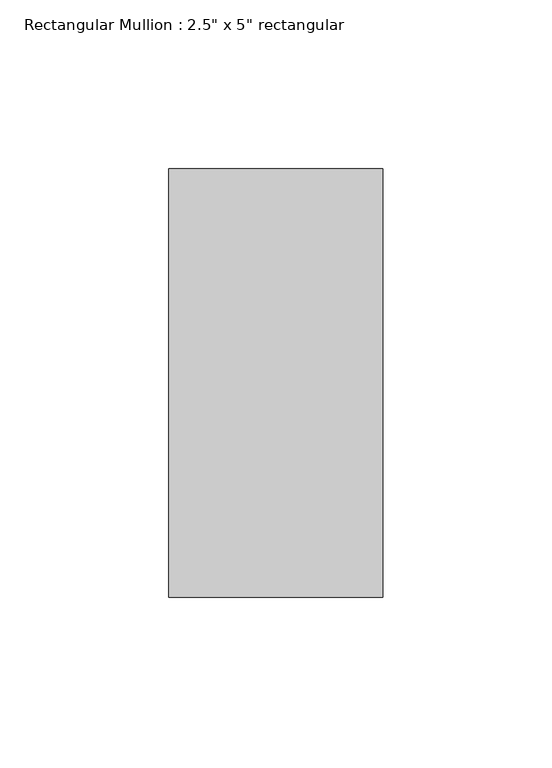
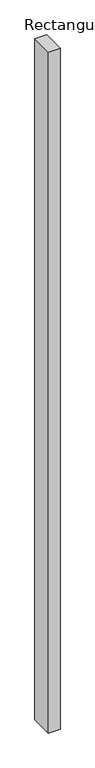
"""IFC4 building model written with IfcOpenShell, lengths in millimetres: member geometry."""

from ifc_helpers import new_model, si_unit, frame, origin, place, context, project, spatial, polyline, outline, extrude, source, transform, mapped, element, save


def member_63be31b3(model_context):
    return source(origin(), model_context, "Body", "SweptSolid", [
        extrude(outline(polyline([(0.0, 63.5), (0.0, -63.5), (-63.5, -63.5), (-63.5, 63.5), (0.0, 63.5)])), frame((0.0, 0.0, -3911.6), z_axis=(0.0, 0.0, 1.0), x_axis=(1.0, 0.0, 0.0)), (0.0, 0.0, 1.0), 3911.6),
    ])


if __name__ == "__main__":
    model = new_model("IFC4")
    model_context = context("Model", 3, world=origin())
    ifc_project = project(units=[si_unit("LENGTHUNIT", "METRE", prefix="MILLI")], contexts=[model_context])
    site = spatial("IfcSite", under=ifc_project)
    building = spatial("IfcBuilding", under=site)
    placement = place(None, origin())
    member_shape = member_63be31b3(model_context)
    element("IfcMember", 1, ObjectType="Rectangular Mullion : 2.5\" x 5\" rectangular", at=placement, inside=building, context=model_context, shape_type="MappedRepresentation", body=[
        mapped(member_shape, transform((0.0, 0.0, 0.0), x_axis=(1.0, 0.0, 0.0), y_axis=(0.0, 1.0, 0.0), z_axis=(0.0, 0.0, 1.0))),
    ])
    save(model, "model.ifc")

# Revit data of these elements
# Type "Rectangular Mullion : 2.5\" x 5\" rectangular"
#   built-in parameter 1007304 = 0.416667 (stored number, unit not read)
#   built-in parameter 1007301 = 0.104167 (stored number, unit not read)
#   built-in parameter 1007300 = 0.104167 (stored number, unit not read)
# Element 1 (IfcMember, "Rectangular Mullion : 2.5\" x 5\" rectangular")
#   Materials on its faces: "Aluminum"
# Materials
#   "Aluminum": class "Metal", colour RGB 247 247 247, transparency 0, Description = "Aluminum 6061", Cost = 0
